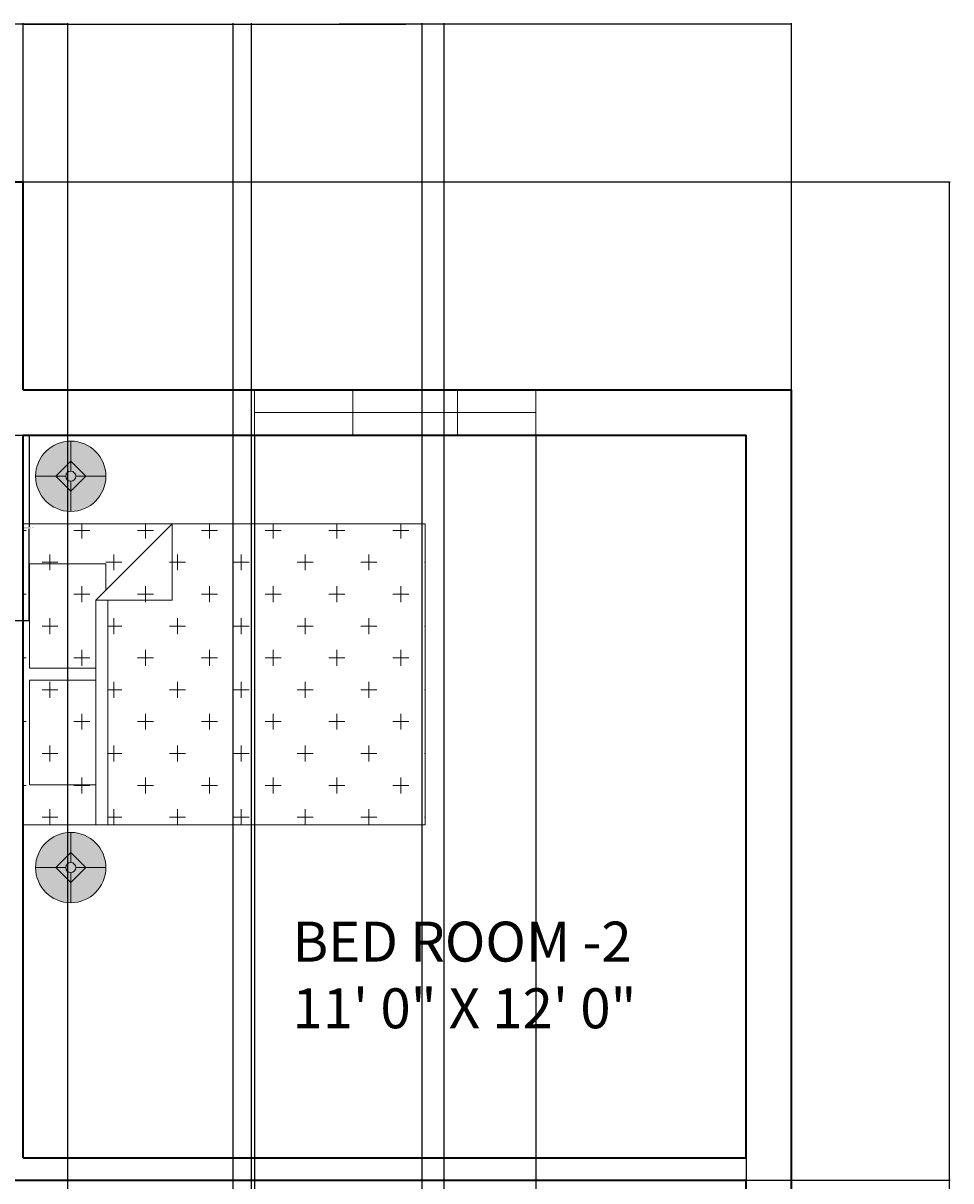
# Model space of a CAD drawing. Units: inches. Extents: x 2284228 to 3635239, y 3024422 to 8351872.
# Tile 7 of 7: x 3635054 to 3635239, y 8351600 to 8351831. Entities that reach past the tile are written whole.
import ezdxf

# ---------------------------------------------------------------- set-up
doc = ezdxf.new("R2010")
doc.units = ezdxf.units.IN
for name, color, linetype, lineweight in [('A-ANNO-DIMS', 2, 'Continuous', 18), ('A-AREA-IDEN', 7, 'Continuous', 18), ('A-FURN', 8, 'Continuous', 18), ('A-FURN-PATT', 9, 'Continuous', 13), ('A-GLAZ', 4, 'Continuous', 18), ('A-WALL', 7, 'Continuous', 35)]:
    doc.layers.add(name, color=color, linetype=linetype, lineweight=lineweight)
doc.styles.get("Standard").update_dxf_attribs({"font": 'arial.ttf'})
doc.dimstyles.get("Standard").update_dxf_attribs({"dimtxt": 0.18, "dimasz": 0.18, "dimexe": 0.18, "dimexo": 0.0625, "dimgap": 0.09, "dimtad": 0, "dimtih": 1, "dimtoh": 1, "dimdec": 4, "dimzin": 0, "dimdsep": 46, "dimtxsty": 'Standard', "dimcen": 0.09, "dimadec": 0, "dimazin": 0, "dimtfac": 1, "dimtdec": 4, "dimtofl": 0, "dimtmove": 0, "dimatfit": 3, "dimfxl": 1, "dimtolj": 1, "dimtzin": 0, "dimarcsym": 0})

# ---------------------------------------------------------------- blocks, each defined once
blk = doc.blocks.new('Bed - Queen')
for p, q in [((0, -80.00003), (0, 0)), ((0, 0), (59.99999, 0)), ((59.99999, 0), (59.99999, -80.00003)), ((7.99999, -1.2), (28.79998, -1.2)), ((7.99999, -14.4), (7.99999, -1.2)), ((28.79998, -1.2), (28.79998, -14.4)), ((31.19999, -1.2), (51.99999, -1.2)), ((31.19999, -14.4), (31.19999, -1.2)), ((51.99999, -1.2), (51.99999, -16.4)), ((0, -14.4), (44.8, -14.4)), ((59.99999, -29.6), (44.8, -14.4)), ((44.8, -14.4), (44.8, -29.6)), ((44.8, -16.8), (0, -16.8)), ((51.99999, -16.4), (46.79936, -16.4)), ((44.8, -29.6), (59.99999, -29.6)), ((59.99999, -80.00003), (0, -80.00003))]:
    blk.add_line(p, q)
blk = doc.blocks.new('Lamp - Table')
for p, q in [((0, 7), (0, 1)), ((0, 3), (-3, 0)), ((3, 0), (0, 3)), ((-1, 0), (-7, 0)), ((-3, 0), (0, -3)), ((0, -3), (3, 0)), ((1, 0), (7, 0)), ((0, -1), (0, -7))]:
    blk.add_line(p, q)
for radius in [7, 1]:
    blk.add_circle((0, 0), radius)
blk = doc.blocks.new('*D38')
at = {"layer": 'A-ANNO-DIMS', "color": 0, "lineweight": -2, "transparency": 16777216}
for p, q in [((3635049.45, 8351748.56), (3635055.11, 8351748.56)), ((3635054.93, 8351748.38), (3635054.93, 8351730.26)), ((3635054.93, 8351711.77), (3635054.93, 8351729.89)), ((3635049.45, 8351711.59), (3635055.11, 8351711.59))]:
    blk.add_line(p, q, dxfattribs=at)
at = {"layer": 'A-ANNO-DIMS', "color": 0, "transparency": 16777216}
for points in [[(3635054.9, 8351748.38), (3635054.96, 8351748.38), (3635054.93, 8351748.56)], [(3635054.9, 8351711.77), (3635054.96, 8351711.77), (3635054.93, 8351711.59)]]:
    blk.add_solid(points, dxfattribs=at)
at = {"layer": 'Defpoints', "color": 0, "transparency": 16777216}
for p in [(3635049.39, 8351748.56), (3635054.93, 8351748.56), (3635049.39, 8351711.59)]:
    blk.add_point(p, dxfattribs=at)
at = {"layer": 'A-ANNO-DIMS', "color": 0, "transparency": 16777216, "insert": (3635054.93, 8351730.08), "char_height": 0.18, "attachment_point": 5}
blk.add_mtext('\\A1;SHOWER 37 TYP.', dxfattribs=at)
blk = doc.blocks.new('*D41')
at = {"layer": 'A-ANNO-DIMS', "color": 0, "lineweight": -2, "transparency": 16777216}
for p, q in [((3635053.81, 8351799.01), (3635238.38, 8351799.01)), ((3635238.2, 8351798.83), (3635238.2, 8351524.72)), ((3635238.2, 8351250.24), (3635238.2, 8351524.36)), ((3635039.81, 8351250.06), (3635238.38, 8351250.06))]:
    blk.add_line(p, q, dxfattribs=at)
at = {"layer": 'A-ANNO-DIMS', "color": 0, "transparency": 16777216}
for points in [[(3635238.17, 8351798.83), (3635238.23, 8351798.83), (3635238.2, 8351799.01)], [(3635238.17, 8351250.24), (3635238.23, 8351250.24), (3635238.2, 8351250.06)]]:
    blk.add_solid(points, dxfattribs=at)
at = {"layer": 'Defpoints', "color": 0, "transparency": 16777216}
for p in [(3635053.75, 8351799.01), (3635238.2, 8351799.01), (3635039.75, 8351250.06)]:
    blk.add_point(p, dxfattribs=at)
at = {"layer": 'A-ANNO-DIMS', "color": 0, "transparency": 16777216, "insert": (3635238.2, 8351524.54), "char_height": 0.18, "attachment_point": 5}
blk.add_mtext('\\A1;549', dxfattribs=at)
blk = doc.blocks.new('*D44')
at = {"layer": 'A-ANNO-DIMS', "color": 0, "lineweight": -2, "transparency": 16777216}
for p, q in [((3635053.75, 8351757.63), (3635053.75, 8351830.64)), ((3635053.93, 8351830.46), (3635129.97, 8351830.46)), ((3635206.57, 8351830.46), (3635130.53, 8351830.46)), ((3635206.75, 8351757.63), (3635206.75, 8351830.64))]:
    blk.add_line(p, q, dxfattribs=at)
at = {"layer": 'A-ANNO-DIMS', "color": 0, "transparency": 16777216}
for points in [[(3635053.93, 8351830.49), (3635053.93, 8351830.43), (3635053.75, 8351830.46)], [(3635206.57, 8351830.49), (3635206.57, 8351830.43), (3635206.75, 8351830.46)]]:
    blk.add_solid(points, dxfattribs=at)
at = {"layer": 'Defpoints', "color": 0, "transparency": 16777216}
for p in [(3635206.75, 8351830.46), (3635053.75, 8351757.56), (3635206.75, 8351757.56)]:
    blk.add_point(p, dxfattribs=at)
at = {"layer": 'A-ANNO-DIMS', "color": 0, "transparency": 16777216, "insert": (3635130.25, 8351830.46), "char_height": 0.18, "attachment_point": 5}
blk.add_mtext('\\A1;153', dxfattribs=at)
blk = doc.blocks.new('*D52')
at = {"layer": 'A-ANNO-DIMS', "color": 0, "lineweight": -2, "transparency": 16777216}
for p, q in [((3635099.83, 8351748.5), (3635099.83, 8351218.43)), ((3635155.88, 8351748.5), (3635155.88, 8351218.43)), ((3635100.01, 8351218.61), (3635127.46, 8351218.61)), ((3635155.7, 8351218.61), (3635128.25, 8351218.61))]:
    blk.add_line(p, q, dxfattribs=at)
at = {"layer": 'A-ANNO-DIMS', "color": 0, "transparency": 16777216}
for points in [[(3635100.01, 8351218.64), (3635100.01, 8351218.58), (3635099.83, 8351218.61)], [(3635155.7, 8351218.64), (3635155.7, 8351218.58), (3635155.88, 8351218.61)]]:
    blk.add_solid(points, dxfattribs=at)
at = {"layer": 'Defpoints', "color": 0, "transparency": 16777216}
for p in [(3635099.83, 8351748.56), (3635155.88, 8351748.56), (3635155.88, 8351218.61)]:
    blk.add_point(p, dxfattribs=at)
at = {"layer": 'A-ANNO-DIMS', "color": 0, "transparency": 16777216, "insert": (3635127.85, 8351218.61), "char_height": 0.18, "attachment_point": 5}
blk.add_mtext('\\A1;56.06', dxfattribs=at)
blk = doc.blocks.new('*D53')
at = {"layer": 'A-ANNO-DIMS', "color": 0, "lineweight": -2, "transparency": 16777216}
for p, q in [((3635155.88, 8351748.5), (3635155.88, 8351218.43)), ((3635197.75, 8351748.5), (3635197.75, 8351218.43)), ((3635156.06, 8351218.61), (3635176.42, 8351218.61)), ((3635197.57, 8351218.61), (3635177.21, 8351218.61))]:
    blk.add_line(p, q, dxfattribs=at)
at = {"layer": 'A-ANNO-DIMS', "color": 0, "transparency": 16777216}
for points in [[(3635156.06, 8351218.64), (3635156.06, 8351218.58), (3635155.88, 8351218.61)], [(3635197.57, 8351218.64), (3635197.57, 8351218.58), (3635197.75, 8351218.61)]]:
    blk.add_solid(points, dxfattribs=at)
at = {"layer": 'Defpoints', "color": 0, "transparency": 16777216}
for p in [(3635155.88, 8351748.56), (3635197.75, 8351748.56), (3635197.75, 8351218.61)]:
    blk.add_point(p, dxfattribs=at)
at = {"layer": 'A-ANNO-DIMS', "color": 0, "transparency": 16777216, "insert": (3635176.82, 8351218.61), "char_height": 0.18, "attachment_point": 5}
blk.add_mtext('\\A1;41.87', dxfattribs=at)
blk = doc.blocks.new('*D57')
at = {"layer": 'A-ANNO-DIMS', "color": 0, "lineweight": -2, "transparency": 16777216}
for p, q in [((3635035.25, 8351378.63), (3635035.25, 8351830.64)), ((3635035.43, 8351830.46), (3635048.63, 8351830.46)), ((3635062.47, 8351830.46), (3635049.28, 8351830.46)), ((3635062.65, 8351378.63), (3635062.65, 8351830.64))]:
    blk.add_line(p, q, dxfattribs=at)
at = {"layer": 'A-ANNO-DIMS', "color": 0, "transparency": 16777216}
for points in [[(3635035.43, 8351830.49), (3635035.43, 8351830.43), (3635035.25, 8351830.46)], [(3635062.47, 8351830.49), (3635062.47, 8351830.43), (3635062.65, 8351830.46)]]:
    blk.add_solid(points, dxfattribs=at)
at = {"layer": 'Defpoints', "color": 0, "transparency": 16777216}
for p in [(3635062.65, 8351830.46), (3635035.25, 8351378.57), (3635062.65, 8351378.57)]:
    blk.add_point(p, dxfattribs=at)
at = {"layer": 'A-ANNO-DIMS', "color": 0, "transparency": 16777216, "insert": (3635048.95, 8351830.46), "char_height": 0.18, "attachment_point": 5}
blk.add_mtext('\\A1;27.4', dxfattribs=at)
blk = doc.blocks.new('*D59')
at = {"layer": 'A-ANNO-DIMS', "color": 0, "lineweight": -2, "transparency": 16777216}
for p, q in [((3635099.24, 8351408.73), (3635099.24, 8351830.64)), ((3635099.42, 8351830.46), (3635115.78, 8351830.46)), ((3635133.07, 8351830.46), (3635116.71, 8351830.46)), ((3635133.25, 8351408.73), (3635133.25, 8351830.64))]:
    blk.add_line(p, q, dxfattribs=at)
at = {"layer": 'A-ANNO-DIMS', "color": 0, "transparency": 16777216}
for points in [[(3635099.42, 8351830.49), (3635099.42, 8351830.43), (3635099.24, 8351830.46)], [(3635133.07, 8351830.49), (3635133.07, 8351830.43), (3635133.25, 8351830.46)]]:
    blk.add_solid(points, dxfattribs=at)
at = {"layer": 'Defpoints', "color": 0, "transparency": 16777216}
for p in [(3635133.25, 8351830.46), (3635099.24, 8351408.67), (3635133.25, 8351408.67)]:
    blk.add_point(p, dxfattribs=at)
at = {"layer": 'A-ANNO-DIMS', "color": 0, "transparency": 16777216, "insert": (3635116.24, 8351830.46), "char_height": 0.18, "attachment_point": 5}
blk.add_mtext('\\A1;34.016', dxfattribs=at)
blk = doc.blocks.new('*D67')
at = {"layer": 'A-ANNO-DIMS', "color": 0, "lineweight": -2, "transparency": 16777216}
for p, q in [((3634972.81, 8351600.06), (3635238.38, 8351600.06)), ((3635238.2, 8351599.88), (3635238.2, 8351588.44)), ((3635238.2, 8351576.63), (3635238.2, 8351588.08)), ((3634972.41, 8351576.45), (3635238.38, 8351576.45))]:
    blk.add_line(p, q, dxfattribs=at)
at = {"layer": 'A-ANNO-DIMS', "color": 0, "transparency": 16777216}
for points in [[(3635238.17, 8351599.88), (3635238.23, 8351599.88), (3635238.2, 8351600.06)], [(3635238.17, 8351576.63), (3635238.23, 8351576.63), (3635238.2, 8351576.45)]]:
    blk.add_solid(points, dxfattribs=at)
at = {"layer": 'Defpoints', "color": 0, "transparency": 16777216}
for p in [(3634972.75, 8351600.06), (3635238.2, 8351600.06), (3634972.35, 8351576.45)]:
    blk.add_point(p, dxfattribs=at)
at = {"layer": 'A-ANNO-DIMS', "color": 0, "transparency": 16777216, "insert": (3635238.2, 8351588.26), "char_height": 0.18, "attachment_point": 5}
blk.add_mtext('\\A1;23.61', dxfattribs=at)
blk = doc.blocks.new('*D78')
at = {"layer": 'A-ANNO-DIMS', "color": 0, "lineweight": -2, "transparency": 16777216}
for p, q in [((3635095.59, 8351556.78), (3635095.59, 8351830.64)), ((3635095.77, 8351830.46), (3635116.37, 8351830.46)), ((3635137.41, 8351830.46), (3635116.81, 8351830.46)), ((3635137.59, 8351556.78), (3635137.59, 8351830.64))]:
    blk.add_line(p, q, dxfattribs=at)
at = {"layer": 'A-ANNO-DIMS', "color": 0, "transparency": 16777216}
for points in [[(3635095.77, 8351830.49), (3635095.77, 8351830.43), (3635095.59, 8351830.46)], [(3635137.41, 8351830.49), (3635137.41, 8351830.43), (3635137.59, 8351830.46)]]:
    blk.add_solid(points, dxfattribs=at)
at = {"layer": 'Defpoints', "color": 0, "transparency": 16777216}
for p in [(3635137.59, 8351830.46), (3635095.59, 8351556.72), (3635137.59, 8351556.72)]:
    blk.add_point(p, dxfattribs=at)
at = {"layer": 'A-ANNO-DIMS', "color": 0, "transparency": 16777216, "insert": (3635116.59, 8351830.46), "char_height": 0.18, "attachment_point": 5}
blk.add_mtext('\\A1;42', dxfattribs=at)

msp = doc.modelspace()

# ---------------------------------------------------------------- hatches: boundary and pattern name
at = {"layer": 'A-FURN-PATT'}
h = msp.add_hatch(color=256, dxfattribs=at)
h.dxf.hatch_style = 1
h.paths.add_polyline_path([(3635063.2289, 8351669.3742, 0.41421356), (3635056.2289, 8351662.3742), (3635060.2289, 8351662.3742), (3635063.2289, 8351665.3742)])
h.paths.add_polyline_path([(3635063.2289, 8351669.3742), (3635063.2289, 8351665.3742), (3635066.2289, 8351662.3742), (3635070.2289, 8351662.3742, 0.41421356)])
h.paths.add_polyline_path([(3635070.2289, 8351662.3742), (3635066.2289, 8351662.3742), (3635063.2289, 8351659.3742), (3635063.2289, 8351655.3742, 0.41421356)])
h.paths.add_polyline_path([(3635063.2289, 8351659.3742), (3635060.2289, 8351662.3742), (3635056.2289, 8351662.3742, 0.41421356), (3635063.2289, 8351655.3742)])
h.paths.add_polyline_path([(3635063.2289, 8351747.3555, 0.41421356), (3635056.2289, 8351740.3555), (3635060.2289, 8351740.3555), (3635063.2289, 8351743.3555)])
h.paths.add_polyline_path([(3635063.2289, 8351747.3555), (3635063.2289, 8351743.3555), (3635066.2289, 8351740.3555), (3635070.2289, 8351740.3555, 0.41421356)])
h.paths.add_polyline_path([(3635070.2289, 8351740.3555), (3635066.2289, 8351740.3555), (3635063.2289, 8351737.3555), (3635063.2289, 8351733.3555, 0.41421356)])
h.paths.add_polyline_path([(3635063.2289, 8351737.3555), (3635060.2289, 8351740.3555), (3635056.2289, 8351740.3555, 0.41421356), (3635063.2289, 8351733.3555)])
h = msp.add_hatch(color=256, dxfattribs=at)
h.dxf.hatch_style = 1
h.paths.add_polyline_path([(3635063.2289, 8351743.3555), (3635060.2289, 8351740.3555), (3635062.2289, 8351740.3555, -0.41421356), (3635063.2289, 8351741.3555)])
h.paths.add_polyline_path([(3635063.2289, 8351743.3555), (3635063.2289, 8351741.3555, -0.41421356), (3635064.2289, 8351740.3555), (3635066.2289, 8351740.3555)])
h.paths.add_polyline_path([(3635066.2289, 8351740.3555), (3635064.2289, 8351740.3555, -0.41421356), (3635063.2289, 8351739.3555), (3635063.2289, 8351737.3555)])
h.paths.add_polyline_path([(3635062.2289, 8351740.3555), (3635060.2289, 8351740.3555), (3635063.2289, 8351737.3555), (3635063.2289, 8351739.3555, -0.41421356)])
h.paths.add_polyline_path([(3635063.2289, 8351665.3742), (3635063.2289, 8351663.3742, -0.41421356), (3635064.2289, 8351662.3742), (3635066.2289, 8351662.3742)])
h.paths.add_polyline_path([(3635063.2289, 8351665.3742), (3635060.2289, 8351662.3742), (3635062.2289, 8351662.3742, -0.41421356), (3635063.2289, 8351663.3742)])
h.paths.add_polyline_path([(3635063.2289, 8351661.3742, -0.41421356), (3635062.2289, 8351662.3742), (3635060.2289, 8351662.3742), (3635063.2289, 8351659.3742)])
h.paths.add_polyline_path([(3635066.2289, 8351662.3742), (3635064.2289, 8351662.3742, -0.41421356), (3635063.2289, 8351661.3742), (3635063.2289, 8351659.3742)])
h = msp.add_hatch(color=256, dxfattribs=at)
h.dxf.hatch_style = 1
h.paths.add_polyline_path([(3635064.2289, 8351740.3555, 1), (3635062.2289, 8351740.3555, 1)])
h.paths.add_polyline_path([(3635062.2289, 8351662.3742, 1), (3635064.2289, 8351662.3742, 1)])
h = msp.add_hatch(dxfattribs=at)
h.set_pattern_fill('CROSS', color=256)
h.paths.add_polyline_path([(3635133.8298, 8351730.8911), (3635083.4298, 8351730.8911), (3635083.4298, 8351715.6911), (3635070.6298, 8351715.6911), (3635070.6298, 8351670.8911), (3635133.8298, 8351670.8911)])
h.paths.add_polyline_path([(3635083.4298, 8351730.8911), (3635068.2298, 8351715.6911), (3635083.4298, 8351715.6911)], flags=17)
h.paths.add_polyline_path([(3635083.4298, 8351730.8911), (3635053.8298, 8351730.8911), (3635053.8298, 8351670.8911), (3635068.2298, 8351670.8911), (3635068.2298, 8351678.8911), (3635055.0298, 8351678.8911), (3635055.0298, 8351699.6911), (3635068.2298, 8351699.6911), (3635068.2298, 8351702.0911), (3635055.0298, 8351702.0911), (3635055.0298, 8351722.8911), (3635070.2298, 8351722.8911), (3635070.2298, 8351717.6911)])
h.paths.add_polyline_path([(3635070.2298, 8351722.8911), (3635055.0298, 8351722.8911), (3635055.0298, 8351702.0911), (3635068.2298, 8351702.0911), (3635068.2298, 8351715.6911), (3635070.2298, 8351717.6911)], flags=17)
h.paths.add_polyline_path([(3635068.2298, 8351699.6911), (3635055.0298, 8351699.6911), (3635055.0298, 8351678.8911), (3635068.2298, 8351678.8911)], flags=17)

# ---------------------------------------------------------------- linework, layer by layer
at = {"layer": 'A-GLAZ'}
for p, q in [((3635099.8261, 8351757.5627), (3635099.8261, 8351748.5627)), ((3635119.4297, 8351757.5627), (3635119.4297, 8351748.5627)), ((3635140.2594, 8351757.5627), (3635140.2594, 8351748.5627)), ((3635155.8817, 8351757.5627), (3635155.8817, 8351748.5627)), ((3635099.8261, 8351753.0627), (3635155.8817, 8351753.0627))]:
    msp.add_line(p, q, dxfattribs=at)
at = {"layer": 'A-WALL'}
for p, q in [((3634896.2525, 8351799.0118), (3635053.7525, 8351799.0118)), ((3635053.7525, 8351757.5627), (3635053.7525, 8351799.0118)), ((3635053.7525, 8351757.5627), (3635206.7525, 8351757.5627)), ((3635206.7525, 8351310.5627), (3635206.7525, 8351757.5627)), ((3635053.7525, 8351604.5627), (3635053.7525, 8351748.5627)), ((3635053.7525, 8351748.5627), (3635197.7525, 8351748.5627)), ((3635197.7525, 8351604.5627), (3635197.7525, 8351748.5627)), ((3635053.7525, 8351604.5627), (3635197.7525, 8351604.5627)), ((3635053.7525, 8351604.5627), (3635197.7525, 8351604.5627)), ((3635009.7751, 8351600.0627), (3635197.7525, 8351600.0627)), ((3635197.7525, 8351467.5627), (3635197.7525, 8351600.0627))]:
    msp.add_line(p, q, dxfattribs=at)

# ---------------------------------------------------------------- block references
at = {"layer": 'A-FURN'}
for p in [(3635063.2289, 8351740.3555), (3635063.2289, 8351662.3742)]:
    msp.add_blockref('Lamp - Table', p, dxfattribs=at)
at = {"layer": 'A-FURN', "rotation": 90}
msp.add_blockref('Bed - Queen', (3635053.8298, 8351670.8911), dxfattribs=at)

# ---------------------------------------------------------------- texts
at = {"layer": 'A-AREA-IDEN', "insert": (3635107.377, 8351651.6046), "char_height": 7.968129, "attachment_point": 1}
msp.add_mtext_dynamic_manual_height_columns('BED ROOM -2\\P11\' 0" X 12\' 0"', width=493.792617, gutter_width=39.8406, heights=[0], dxfattribs=at)

# ---------------------------------------------------------------- dimensions: what is measured, and where the dimension line sits
at = {"layer": 'A-ANNO-DIMS'}
for base, p1, p2, override, picture, middle in [((3635062.6524, 8351830.4618), (3635035.2525, 8351378.5661), (3635062.6524, 8351378.5661), {"dimdec": 1, "dimlfac": 1, "dimrnd": 0, "dimzin": 0, "dimdsep": 46, "dimlunit": 2}, '*D57', (3635048.9524, 8351830.4618)), ((3635206.7525, 8351830.4618), (3635053.7525, 8351757.5627), (3635206.7525, 8351757.5627), {"dimdec": 0, "dimlfac": 1, "dimrnd": 0, "dimzin": 0, "dimdsep": 46, "dimlunit": 2}, '*D44', (3635130.2525, 8351830.4618)), ((3635137.5898, 8351830.4618), (3635095.5898, 8351556.7209), (3635137.5898, 8351556.7209), {"dimdec": 0, "dimlfac": 1, "dimrnd": 0, "dimzin": 0, "dimdsep": 46, "dimlunit": 2}, '*D78', (3635116.5898, 8351830.4618)), ((3635133.2525, 8351830.4618), (3635099.2364, 8351408.6677), (3635133.2525, 8351408.6677), {"dimdec": 3, "dimlfac": 1, "dimrnd": 0, "dimzin": 0, "dimdsep": 46, "dimlunit": 2}, '*D59', (3635116.2444, 8351830.4618)), ((3635155.8817, 8351218.6127), (3635099.8261, 8351748.5627), (3635155.8817, 8351748.5627), {"dimdec": 2, "dimlfac": 1, "dimrnd": 0, "dimzin": 0, "dimdsep": 46, "dimlunit": 2}, '*D52', (3635127.8539, 8351218.6127)), ((3635197.7525, 8351218.6127), (3635155.8817, 8351748.5627), (3635197.7525, 8351748.5627), {"dimdec": 2, "dimlfac": 1, "dimrnd": 0, "dimzin": 0, "dimdsep": 46, "dimlunit": 2}, '*D53', (3635176.8171, 8351218.6127))]:
    dim = msp.add_linear_dim(base=base, p1=p1, p2=p2, dimstyle='Standard', override=override, dxfattribs=at)
    dim.commit()
    dim.dimension.update_dxf_attribs({"geometry": picture, "text_midpoint": middle})
for base, p1, p2, override, picture, middle in [((3635238.2025, 8351799.0118), (3635039.7525, 8351250.0627), (3635053.7525, 8351799.0118), {"dimdec": 0, "dimlfac": 1, "dimrnd": 0, "dimzin": 0, "dimdsep": 46, "dimlunit": 2}, '*D41', (3635238.2025, 8351524.5372)), ((3635238.2025, 8351600.0627), (3634972.3485, 8351576.4517), (3634972.7525, 8351600.0627), {"dimdec": 2, "dimlfac": 1, "dimrnd": 0, "dimzin": 0, "dimdsep": 46, "dimlunit": 2}, '*D67', (3635238.2025, 8351588.2572))]:
    dim = msp.add_linear_dim(base=base, p1=p1, p2=p2, angle=90, dimstyle='Standard', override=override, dxfattribs=at)
    dim.commit()
    dim.dimension.update_dxf_attribs({"geometry": picture, "text_midpoint": middle})
dim = msp.add_linear_dim(base=(3635054.9328, 8351748.5627), p1=(3635049.3867, 8351711.5887), p2=(3635049.3867, 8351748.5627), angle=90, text='SHOWER <> TYP.', dimstyle='Standard', override={"dimdec": 0, "dimlfac": 1, "dimrnd": 0, "dimzin": 0, "dimdsep": 46, "dimlunit": 2}, dxfattribs=at)
dim.commit()
dim.dimension.update_dxf_attribs({"geometry": '*D38', "text_midpoint": (3635054.9328, 8351730.0757)})

doc.saveas('drawing.dxf')
